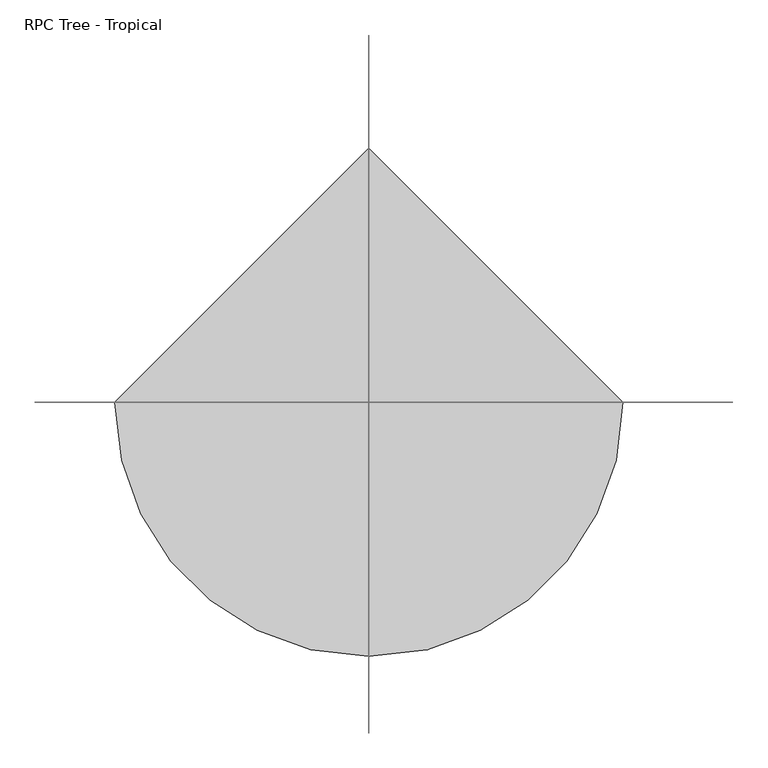
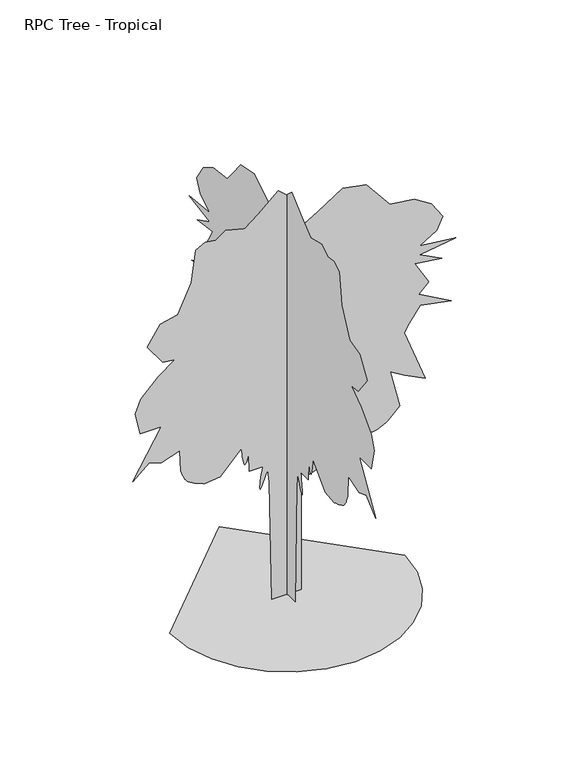
"""IFC4 building model written with IfcOpenShell, lengths in millimetres: geographic element geometry, RPC Tree - Tropical."""

from ifc_helpers import new_model, si_unit, origin, place, context, project, spatial, triangles, source, transform, mapped, element, save


def rpc_tree_tropical_d7a905c7(model_context):
    return source(origin(), model_context, "Body", "Tessellation", [
        triangles([(-0.2241189, -80.6803134, 0.0560704), (-0.2241181, -93.4507094, 708.3955685), (-0.2241176, -102.9729479, 784.5729681), (-0.2241171, -112.4304103, 759.6428038), (-0.2241163, -121.4992608, 736.1299221), (-0.2241158, -129.7908604, 715.4466642), (-0.2241156, -136.916343, 699.0127836), (-0.2241151, -142.4870876, 688.2406214), (-0.2241151, -146.1147278, 684.5474602), (-0.2241148, -147.4101338, 689.3505827), (-0.2241148, -146.9475984, 700.5392893), (-0.2241151, -145.6519381, 714.7252693), (-0.2241151, -143.662352, 731.4105881), (-0.2241153, -141.1175219, 750.0923693), (-0.2241156, -138.1563745, 770.2752216), (-0.2241156, -134.9173553, 791.458885), (-0.2241158, -131.5396545, 813.1404104), (-0.2241113, -207.7180624, 813.1404104), (-0.224111, -210.8920511, 914.7103008), (-0.2241108, -214.9636775, 900.580204), (-0.2241105, -218.9799477, 887.367057), (-0.2241105, -222.88496, 875.9827955), (-0.2241103, -226.6235945, 867.3493109), (-0.22411, -230.1402221, 862.3810095), (-0.2241097, -233.3789961, 861.9923704), (-0.2241095, -236.2847599, 867.1003435), (-0.2241095, -238.9129061, 876.4653969), (-0.2241092, -241.3744383, 887.9944897), (-0.2241092, -243.6972616, 901.3295042), (-0.224109, -245.9088635, 916.1097794), (-0.224109, -248.0373855, 931.9696398), (-0.2241087, -250.1102786, 948.5533659), (-0.2241087, -252.1552483, 965.4977531), (-0.2241016, -372.7715778, 838.5329012), (-0.2240963, -461.6464946, 829.010372), (-0.224095, -479.2563572, 835.8125004), (-0.224094, -496.4217339, 842.6147015), (-0.2240932, -512.6981023, 849.4168299), (-0.2240922, -527.64352, 856.2164148), (-0.2240914, -540.8134646, 863.0185432), (-0.2240907, -551.7608706, 869.8206717), (-0.2240902, -560.0413244, 876.6228727), (-0.2240899, -566.4726179, 884.1641275), (-0.2240897, -572.238436, 893.0389492), (-0.2240892, -577.4480018, 903.0236595), (-0.2240889, -582.2155887, 913.8974871), (-0.2240887, -586.6479126, 925.4367537), (-0.2240884, -590.8567037, 937.4204699), (-0.2240881, -594.9562717, 949.6252481), (-0.2240879, -601.3062839, 1073.4150759), (-0.2240815, -706.0511621, 1038.5001286), (-0.2240775, -775.8810568, 1063.8925467), (-0.2240719, -867.928418, 981.3677147), (-0.2240815, -706.0511621, 1254.3398609), (-0.2240744, -826.6659657, 1254.3398609), (-0.2240727, -855.233408, 1381.3021694), (-0.2240747, -823.4909414, 1460.6545933), (-0.2240805, -725.0961479, 1562.224411), (-0.2240861, -629.8712191, 1632.0567764), (-0.2240821, -699.7011137, 1641.5768349), (-0.224077, -785.4035133, 1759.0190849), (-0.2240813, -712.3985945, 1873.2865288), (-0.2240871, -614.0012575, 1895.5039227), (-0.2240917, -537.8238579, 2060.5586735), (-0.2240932, -512.4314034, 2247.8284927), (-0.2240963, -458.4714704, 2276.3959351), (-0.2240998, -398.1640686, 2266.8734058), (-0.2241034, -341.0291113, 2308.1358582), (-0.2241097, -233.1107712, 2279.5708866), (-0.2241143, -156.9326267, 2339.8783974), (-0.2241212, -42.6652782, 2438.2757343), (-0.2241265, 46.2093524, 2358.9233105), (-0.2241265, 46.2093524, 2263.6984543), (-0.2241298, 103.3427746, 2190.6960789), (-0.2241346, 182.6954255, 2235.1334827), (-0.224143, 322.3549604, 2327.1809166), (-0.2241509, 455.6672811, 2301.7884258), (-0.2241557, 538.1921494, 2200.2186081), (-0.2241588, 588.979638, 2136.7361458), (-0.2241672, 728.6394636, 2117.6910873), (-0.224173, 827.0368006, 2057.3837219), (-0.2241768, 890.5167194, 1958.986385), (-0.2241748, 855.6017721, 1889.1564903), (-0.2241689, 760.3793867, 1828.8489796), (-0.2241811, 963.5216383, 1806.6315857), (-0.2241689, 760.3793867, 1774.8890465), (-0.2241763, 884.1692144, 1711.4067295), (-0.2241674, 731.8118717, 1730.4516426), (-0.224172, 811.1642956, 1593.9668049), (-0.2241687, 754.0318817, 1540.0068718), (-0.2241796, 938.1291475, 1435.2621025), (-0.2241692, 763.5544109, 1470.1769772), (-0.2241654, 700.0719486, 1384.477121), (-0.2241636, 671.5045063, 1336.8647655), (-0.224171, 792.1193098, 1022.630167), (-0.2241639, 674.6795305, 1079.7650517), (-0.224159, 592.1520824, 1130.5500332), (-0.2241621, 646.1120155, 908.3627958), (-0.2241583, 579.4571451, 841.7079254), (-0.2241575, 566.5462689, 834.2758209), (-0.2241567, 553.721761, 827.1511105), (-0.224156, 541.0623593, 820.6359558), (-0.2241552, 528.6518887, 815.0378237), (-0.2241544, 516.5766809, 810.6613466), (-0.2241537, 504.9155105, 807.8089771), (-0.2241532, 493.7572526, 806.7929054), (-0.2241524, 482.6879065, 807.6260668), (-0.2241519, 471.2883479, 809.9577559), (-0.2241511, 459.6093733, 813.5392233), (-0.2241504, 447.7094456, 818.1188129), (-0.2241496, 435.6418682, 823.4503189), (-0.2241489, 423.4625244, 829.2796143), (-0.2241481, 411.2298409, 835.357877), (-0.2241481, 407.7779803, 839.4116993), (-0.2241478, 404.0213056, 843.2979446), (-0.2241476, 399.6524952, 846.8514341), (-0.2241471, 394.3692784, 849.9070616), (-0.2241468, 387.8643339, 852.2946339), (-0.2241463, 379.8302676, 853.8491175), (-0.2241458, 369.9674249, 854.4028627), (-0.224145, 357.1403735, 855.883659), (-0.224144, 340.8157522, 860.0289728), (-0.2241428, 321.5777186, 866.3967527), (-0.2241415, 300.0079778, 874.5400057), (-0.2241402, 276.6881621, 884.0168255), (-0.2241387, 252.2014664, 894.3800737), (-0.2241372, 227.1326114, 905.1877716), (-0.2241349, 185.8694142, 857.577887), (-0.2241349, 185.8694142, 778.2254631), (-0.2241362, 208.0876256, 702.0480635), (-0.2241316, 131.9097354, 676.6556454), (-0.2241288, 87.4725496, 800.4429296), (-0.2241293, 88.096376, 0.0), (-666.8181644, -2.5e-06, 0.2128606), (-649.2007078, -152.6793797, 0.2128611), (-599.0329851, -292.8908795, 0.2128626), (-520.3257617, -416.61723, 0.2128649), (-417.1023385, -519.8431603, 0.2128679), (-293.3760243, -598.5478403, 0.2128717), (-153.1642702, -648.715563, 0.2128758), (-0.4850755, -666.3330196, 0.2128804), (152.1942349, -648.715563, 0.2128849), (292.4057347, -598.5478403, 0.212889), (416.1320852, -519.8406169, 0.2128928), (519.3580155, -416.61723, 0.2128959), (598.0626955, -292.8908795, 0.2128981), (648.2304182, -152.6791254, 0.2128997), (665.8478748, 5.82e-05, 0.2129002), (-0.4851924, 666.3330196, 0.2128804), (-89.341994, 0.0001455, 0.1894216), (-102.11239, 0.0001057, 708.5276825), (-111.6346285, 9.96e-05, 784.7075529), (-121.0920909, 0.0001025, 759.7773886), (-130.1609414, 0.0001023, 736.2619635), (-138.4522867, 0.0001051, 715.581249), (-145.5777693, 0.000105, 699.144825), (-151.1487682, 0.0001048, 688.3726627), (-154.7761631, 0.0001075, 684.682045), (-156.0718144, 0.0001043, 689.4852402), (-155.6090338, 0.0001041, 700.6714033), (-154.3136187, 0.0001037, 714.8573833), (-152.3240326, 0.0001034, 731.5426294), (-149.7792025, 0.0001031, 750.2269541), (-146.8178008, 9.98e-05, 770.4098791), (-143.5790359, 9.95e-05, 791.590999), (-140.2013351, 9.92e-05, 813.2725245), (-216.3794887, 9.82e-05, 813.2725245), (-219.5534773, 9.2e-05, 914.8448856), (-223.6253582, 9.2e-05, 900.7147888), (-227.6413739, 9.5e-05, 887.4991711), (-231.5466406, 9.5e-05, 876.1173803), (-235.2852751, 9.49e-05, 867.4838957), (-238.8016665, 9.47e-05, 862.5131235), (-242.0406767, 9.44e-05, 862.1244844), (-244.9461861, 9.4e-05, 867.2324575), (-247.5745867, 9.35e-05, 876.5974382), (-250.0361189, 9.29e-05, 888.1290745), (-252.358706, 9.23e-05, 901.464089), (-254.5697811, 9.17e-05, 916.2418934), (-256.6983031, 9.1e-05, 932.1042246), (-258.7709418, 9.04e-05, 948.6854073), (-260.8156571, 8.97e-05, 965.6297945), (-381.4330041, 9.73e-05, 838.667486), (-470.3079208, 9.84e-05, 829.1450294), (-487.9177835, 9.66e-05, 835.9446144), (-505.0831601, 9.78e-05, 842.7467428), (-521.3595285, 9.61e-05, 849.5488712), (-536.3049462, 9.46e-05, 856.3510723), (-549.4748909, 9.61e-05, 863.1532007), (-560.4222968, 9.49e-05, 869.9527857), (-568.7027507, 9.4e-05, 876.7549141), (-575.1340442, 9.32e-05, 884.2962416), (-580.8998623, 9.24e-05, 893.1709906), (-586.109428, 9.17e-05, 903.1557735), (-590.8770149, 9.38e-05, 914.0295284), (-595.3093389, 9.31e-05, 925.568795), (-599.5181299, 9.23e-05, 937.5525839), (-603.617698, 9.16e-05, 949.759833), (-609.9677101, 8.15e-05, 1073.5496607), (-714.7125521, 8.49e-05, 1038.6347134), (-784.5424467, 8.37e-05, 1064.0272041), (-876.5898079, 8.96e-05, 981.4997561), (-714.7125521, 7.26e-05, 1254.4719749), (-835.3274282, 7.35e-05, 1254.4719749), (-863.8948706, 6.42e-05, 1381.4367542), (-832.152404, 5.89e-05, 1460.7891781), (-733.7575378, 5.3e-05, 1562.3589958), (-638.532609, 5.06e-05, 1632.1888905), (-708.3625763, 4.99e-05, 1641.7114197), (-794.0649759, 4.17e-05, 1759.1538151), (-721.0600571, 3.61e-05, 1873.4184975), (-622.6626474, 3.25e-05, 1895.6385075), (-546.4852841, 2.27e-05, 2060.6907875), (-521.0928297, 1.36e-05, 2247.9630775), (-467.1328966, 1.17e-05, 2276.5305199), (-406.8254949, 1.15e-05, 2267.0079906), (-349.6905375, 9.6e-06, 2308.270443), (-241.7724518, 1.13e-05, 2279.7030006), (-165.5940529, 7.6e-06, 2340.0103661), (-51.3267045, 3e-07, 2438.4078484), (37.5476695, 7.7e-06, 2359.0554245), (37.5476695, 1.34e-05, 2263.8330391), (94.6810849, 1.78e-05, 2190.8281929), (174.0337449, 1.48e-05, 2235.2655968), (313.6935342, 7e-06, 2327.3155014), (447.0058548, 1.09e-05, 2301.9230106), (529.5307231, 1.55e-05, 2200.3505768), (580.3182117, 1.9e-05, 2136.8682598), (719.978001, 2.04e-05, 2117.8258175), (818.3728672, 2.51e-05, 2057.515836), (881.8552568, 3.08e-05, 1959.1209698), (846.9403095, 3.56e-05, 1889.2910751), (751.7179241, 3.77e-05, 1828.9837097), (954.8601757, 3.9e-05, 1806.7636997), (751.7179241, 4.22e-05, 1775.0237766), (875.5077518, 4.35e-05, 1711.5413143), (723.1504818, 4.39e-05, 1730.5862274), (802.502833, 5.21e-05, 1594.0989189), (745.3704918, 5.45e-05, 1540.1416019), (929.4676849, 6.24e-05, 1435.3942165), (754.8929483, 6.03e-05, 1470.3117073), (691.4105587, 6.3e-05, 1384.609235), (662.8430437, 6.77e-05, 1336.9993504), (783.4579199, 8.5e-05, 1022.7647518), (666.0180679, 8.15e-05, 1079.8971657), (583.4906562, 7.85e-05, 1130.6820745), (637.4506256, 9.28e-05, 908.4973806), (570.7957189, 9.76e-05, 841.8399668), (557.8848427, 9.67e-05, 834.4104784), (545.0603348, 9.87e-05, 827.2831518), (532.4009331, 9.77e-05, 820.7706133), (519.9904624, 9.97e-05, 815.169865), (507.9152547, 9.88e-05, 810.7934607), (496.2540842, 9.78e-05, 807.9435619), (485.0932829, 9.98e-05, 806.9250195), (474.0264802, 9.87e-05, 807.7581808), (462.6269217, 9.77e-05, 810.0898699), (450.947947, 9.94e-05, 813.6712646), (439.0480193, 9.82e-05, 818.2534704), (426.980442, 9.7e-05, 823.5823603), (414.8010982, 9.86e-05, 829.4117283), (402.5684146, 9.74e-05, 835.4924618), (399.1165541, 9.69e-05, 839.5463568), (395.3598793, 9.65e-05, 843.4325294), (390.9910689, 9.6e-05, 846.9860189), (385.7078522, 9.54e-05, 850.0391029), (379.2029077, 9.48e-05, 852.4267479), (371.1688414, 9.69e-05, 853.9812315), (361.3059986, 9.6e-05, 854.5374475), (348.4789473, 9.48e-05, 856.0183165), (332.154326, 9.62e-05, 860.1635576), (312.9162924, 9.43e-05, 866.5288668), (291.3465516, 9.5e-05, 874.6721197), (268.0267359, 9.56e-05, 884.1488668), (243.5397858, 9.31e-05, 894.5146585), (218.4709308, 9.34e-05, 905.3224291), (177.2077336, 9.7e-05, 857.7099283), (177.2077336, 9.94e-05, 778.3575771), (199.4261993, 0.0001036, 702.1801775), (123.2483092, 0.0001063, 676.7876867), (78.8108599, 9.87e-05, 800.5775145), (79.4346863, 0.0001459, 0.1333563)], [[85, 84, 86], [53, 52, 54], [91, 90, 92], [87, 86, 88], [95, 94, 96], [96, 94, 97], [9, 8, 10], [52, 51, 54], [51, 50, 54], [1, 133, 2], [133, 132, 2], [2, 132, 3], [131, 130, 132], [130, 129, 132], [129, 128, 132], [18, 17, 19], [71, 70, 72], [72, 70, 73], [10, 8, 11], [8, 7, 11], [11, 7, 12], [7, 6, 12], [12, 6, 13], [6, 5, 13], [13, 5, 14], [5, 4, 14], [14, 4, 15], [4, 3, 15], [15, 3, 16], [16, 3, 17], [55, 54, 56], [89, 88, 90], [56, 54, 57], [57, 54, 58], [61, 60, 62], [62, 60, 63], [60, 59, 63], [25, 24, 26], [24, 23, 26], [26, 23, 27], [23, 22, 27], [27, 22, 28], [22, 21, 28], [28, 21, 29], [21, 20, 29], [29, 20, 30], [20, 19, 30], [30, 19, 31], [82, 81, 83], [83, 81, 84], [81, 80, 84], [80, 79, 84], [70, 69, 73], [98, 97, 99], [31, 19, 32], [99, 97, 100], [58, 54, 59], [100, 97, 101], [101, 97, 102], [102, 97, 103], [103, 97, 104], [104, 97, 105], [105, 97, 106], [106, 97, 107], [107, 97, 108], [108, 97, 109], [109, 97, 110], [110, 97, 111], [111, 97, 112], [112, 97, 113], [113, 97, 114], [114, 97, 115], [115, 97, 116], [116, 97, 117], [117, 97, 118], [118, 97, 119], [119, 97, 120], [120, 97, 121], [121, 97, 122], [122, 97, 123], [123, 97, 124], [124, 97, 125], [125, 97, 126], [126, 97, 127], [65, 64, 66], [66, 64, 67], [68, 67, 69], [67, 64, 69], [3, 132, 17], [73, 69, 74], [69, 64, 74], [64, 63, 74], [63, 59, 74], [17, 132, 19], [132, 128, 19], [128, 127, 19], [92, 90, 93], [76, 75, 77], [77, 75, 78], [78, 75, 79], [79, 75, 84], [75, 74, 84], [74, 59, 84], [84, 59, 86], [86, 59, 88], [88, 59, 90], [90, 59, 93], [93, 59, 94], [94, 59, 97], [97, 59, 127], [127, 59, 19], [32, 19, 33], [19, 59, 33], [59, 54, 33], [54, 50, 33], [33, 50, 34], [50, 49, 34], [34, 49, 35], [35, 49, 36], [36, 49, 37], [49, 48, 37], [37, 48, 38], [48, 47, 38], [38, 47, 39], [47, 46, 39], [39, 46, 40], [46, 45, 40], [45, 44, 40], [40, 44, 41], [44, 43, 41], [41, 43, 42], [148, 149, 134], [147, 148, 134], [147, 134, 135], [146, 147, 135], [146, 135, 136], [146, 136, 137], [145, 146, 137], [144, 145, 137], [144, 137, 138], [144, 138, 139], [144, 139, 140], [144, 140, 141], [144, 141, 142], [144, 142, 143], [233, 234, 235], [201, 202, 203], [239, 240, 241], [235, 236, 237], [243, 244, 245], [243, 245, 246], [157, 158, 159], [200, 201, 203], [199, 200, 203], [282, 150, 151], [281, 282, 151], [281, 151, 152], [279, 280, 281], [278, 279, 281], [277, 278, 281], [166, 167, 168], [219, 220, 221], [219, 221, 222], [157, 159, 160], [156, 157, 160], [156, 160, 161], [155, 156, 161], [155, 161, 162], [154, 155, 162], [154, 162, 163], [153, 154, 163], [153, 163, 164], [152, 153, 164], [152, 164, 165], [152, 165, 166], [203, 204, 205], [237, 238, 239], [203, 205, 206], [203, 206, 207], [209, 210, 211], [209, 211, 212], [208, 209, 212], [173, 174, 175], [172, 173, 175], [172, 175, 176], [171, 172, 176], [171, 176, 177], [170, 171, 177], [170, 177, 178], [169, 170, 178], [169, 178, 179], [168, 169, 179], [168, 179, 180], [230, 231, 232], [230, 232, 233], [229, 230, 233], [228, 229, 233], [218, 219, 222], [246, 247, 248], [168, 180, 181], [246, 248, 249], [203, 207, 208], [246, 249, 250], [246, 250, 251], [246, 251, 252], [246, 252, 253], [246, 253, 254], [246, 254, 255], [246, 255, 256], [246, 256, 257], [246, 257, 258], [246, 258, 259], [246, 259, 260], [246, 260, 261], [246, 261, 262], [246, 262, 263], [246, 263, 264], [246, 264, 265], [246, 265, 266], [246, 266, 267], [246, 267, 268], [246, 268, 269], [246, 269, 270], [246, 270, 271], [246, 271, 272], [246, 272, 273], [246, 273, 274], [246, 274, 275], [246, 275, 276], [213, 214, 215], [213, 215, 216], [216, 217, 218], [213, 216, 218], [281, 152, 166], [218, 222, 223], [213, 218, 223], [212, 213, 223], [208, 212, 223], [281, 166, 168], [277, 281, 168], [276, 277, 168], [239, 241, 242], [224, 225, 226], [224, 226, 227], [224, 227, 228], [224, 228, 233], [223, 224, 233], [208, 223, 233], [208, 233, 235], [208, 235, 237], [208, 237, 239], [208, 239, 242], [208, 242, 243], [208, 243, 246], [208, 246, 276], [208, 276, 168], [168, 181, 182], [208, 168, 182], [203, 208, 182], [199, 203, 182], [199, 182, 183], [198, 199, 183], [198, 183, 184], [198, 184, 185], [198, 185, 186], [197, 198, 186], [197, 186, 187], [196, 197, 187], [196, 187, 188], [195, 196, 188], [195, 188, 189], [194, 195, 189], [193, 194, 189], [193, 189, 190], [192, 193, 190], [192, 190, 191]], closed=False),
    ])


if __name__ == "__main__":
    model = new_model("IFC4")
    model_context = context("Model", 3, world=origin())
    ifc_project = project(units=[si_unit("LENGTHUNIT", "METRE", prefix="MILLI")], contexts=[model_context])
    site = spatial("IfcSite", under=ifc_project)
    building = spatial("IfcBuilding", under=site)
    placement = place(None, origin())
    rpc_tree_tropical_shape = rpc_tree_tropical_d7a905c7(model_context)
    element("IfcGeographicElement", 1, ObjectType="RPC Tree - Tropical", at=placement, inside=building, context=model_context, shape_type="MappedRepresentation", body=[
        mapped(rpc_tree_tropical_shape, transform((0.0, 0.0, 0.0), x_axis=(1.0, 0.0, 0.0), y_axis=(0.0, 1.0, 0.0), z_axis=(0.0, 0.0, 1.0))),
    ])
    save(model, "model.ifc")

# Revit data of these elements
# Type "RPC Tree - Tropical"
#   built-in parameter 1005198 = "{2, 15},{39, RPC-16-G2MF-J1Q0-CAN1-N000-ST1L-LVER-AU},{1, 0},{1, 0},{2, 13},{1, 8},{5, Color},{1, 0},{1, 0},{3, 0.8},{3, 0.8},{3, 0.8},{1, 8},{7, BBoxMin},{1, 0},{1, 0},{1, 0},{1, 0},{1, 0},{1, 8},{7, BBoxMax},{1, 0},{1, 0},{1, 0},{1, 0},{1, 0},{2, 11},{9, RPCTypeId},{1, 0},{1, 0},{39, RPC-16-G2MF-J1Q0-CAN1-N000-ST1L-LVER-AU},{1, 6},{14, RPCPlantHeight},{1, 0},{1, 0},{1, 8},{2, 11},{7, keyword},{1, 0},{1, 0},{35, :RPCs:Trees [Tropical]:Geometry:RPC},{2, 11},{8, category},{1, 0},{1, 0},{16, Trees [Tropical]},{2, 11},{12, LocalizedUID},{1, 0},{1, 0},{13, Windmill Palm},{2, 14},{6, Height},{1, 0},{1, 0},{1, 8},{1, 2},{16, Cast Reflections},{1, 0},{1, 0},{1, 0},{1, 2},{12, Cast Shadows},{1, 0},{1, 0},{1, 1},{1, 2},{9, Lock View},{1, 0},{1, 0},{1, 0},{1, 4},{5, ViewC},{1, 0},{1, 0},{1, 0},{21, assetlibrary_base.fbx},{1, 5},"
#   built-in parameter 1005195 = "RPC-16-G2MF-J1Q0-CAN1-N000-ST1L-LVER-AU"
#   Assembly Code = "G2050500"
#   Height = 8' - 0"
#   Plan Symbol = element 361270
#   Default Elevation = 0
